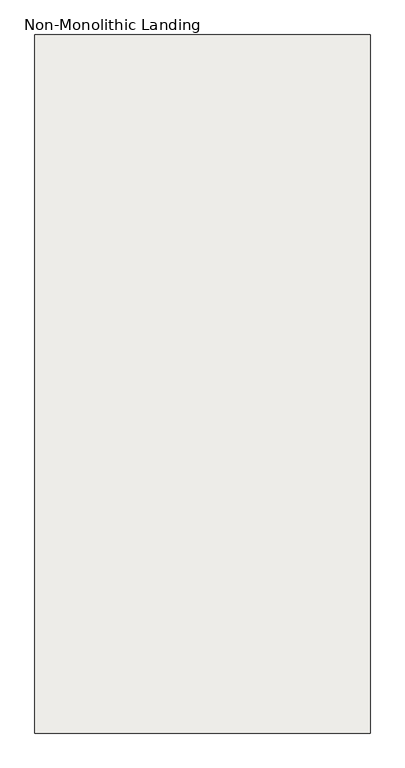
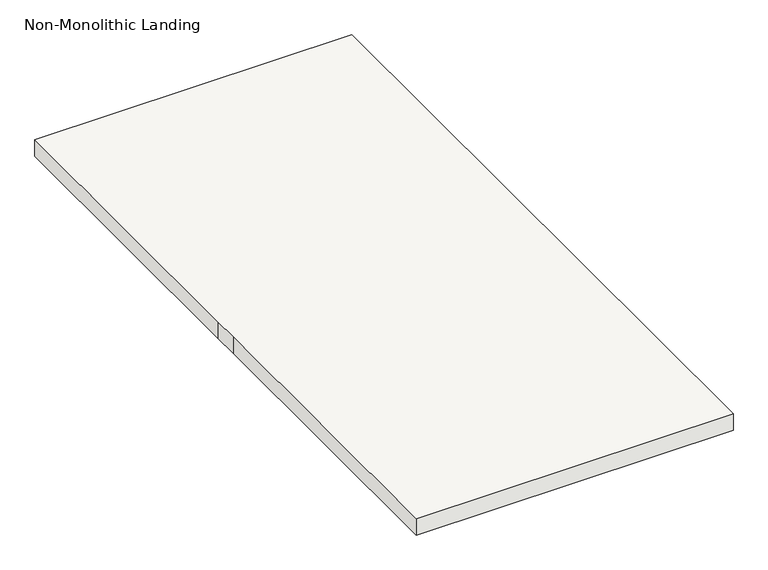
"""IFC4 building model written with IfcOpenShell, lengths in millimetres: slab geometry, Non-Monolithic Landing."""

from ifc_helpers import new_model, si_unit, frame, origin, place, context, project, spatial, polyline, outline, extrude, source, transform, mapped, element, save


def non_monolithic_landing_e1259e21(model_context):
    return source(origin(), model_context, "Body", "SweptSolid", [
        extrude(outline(polyline([(-7545.4329612, -2123.2421603), (-6631.0329612, -2123.2421603), (-6631.0329612, -4028.2421603), (-7545.4329612, -4028.2421603), (-7545.4329612, -3113.8421603), (-7545.4329612, -3037.6421603), (-7545.4329612, -2123.2421603)])), frame((0.0, 0.0, 4750.6), z_axis=(0.0, 0.0, 1.0), x_axis=(1.0, 0.0, 0.0)), (0.0, 0.0, 1.0), 50.0),
    ])


if __name__ == "__main__":
    model = new_model("IFC4")
    model_context = context("Model", 3, world=origin())
    ifc_project = project(units=[si_unit("LENGTHUNIT", "METRE", prefix="MILLI")], contexts=[model_context])
    site = spatial("IfcSite", under=ifc_project)
    building = spatial("IfcBuilding", under=site)
    placement = place(None, origin())
    non_monolithic_landing_shape = non_monolithic_landing_e1259e21(model_context)
    element("IfcSlab", 1, ObjectType="Non-Monolithic Landing", at=placement, inside=building, context=model_context, shape_type="MappedRepresentation", body=[
        mapped(non_monolithic_landing_shape, transform((0.0, 0.0, 0.0), x_axis=(1.0, 0.0, 0.0), y_axis=(0.0, 1.0, 0.0), z_axis=(0.0, 0.0, 1.0))),
    ])
    save(model, "model.ifc")
